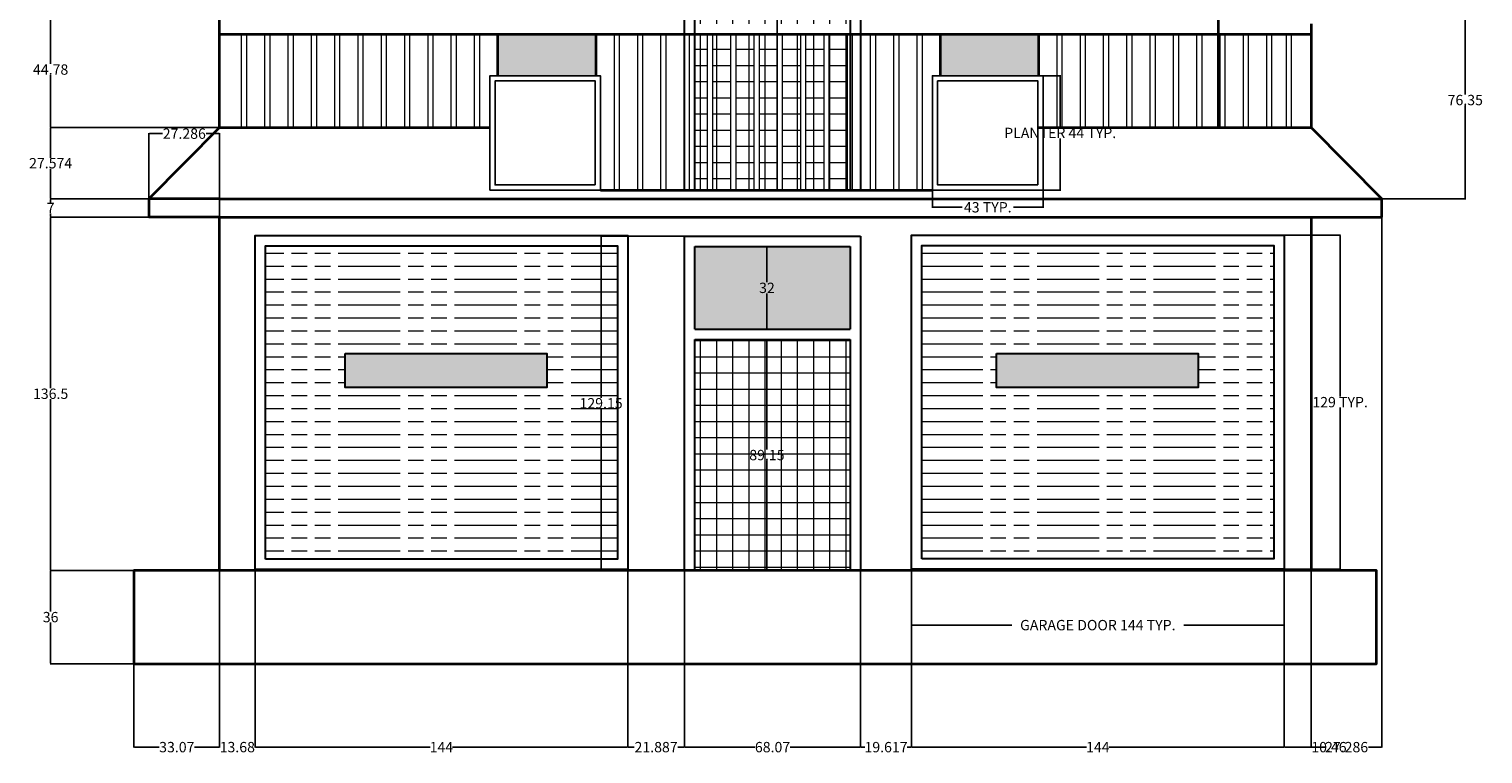
# Model space of a CAD drawing. Units: inches. Extents: x 1366 to 1929, y 372 to 1068.
# Tile 1 of 4: x 1366 to 1927, y 372 to 652. Entities that reach past the tile are written whole.
import ezdxf

# ---------------------------------------------------------------- set-up
doc = ezdxf.new("R2010")
doc.units = ezdxf.units.IN
doc.header["$MEASUREMENT"] = 0
for name, color, linetype, lineweight in [('A-ANNO-DIMS', 2, 'Continuous', 18), ('A-DOOR', 4, 'Continuous', 30), ('A-ELEV', 7, 'Continuous', 35), ('A-ELEV-PATT', 252, 'Continuous', 13), ('A-ELEV-PLNT', 3, 'Continuous', 25), ('A-ELEV-RAIL', 8, 'Continuous', 18)]:
    doc.layers.add(name, color=color, linetype=linetype, lineweight=lineweight)
doc.styles.get("Standard").update_dxf_attribs({"font": 'arial.ttf'})
doc.dimstyles.get("Standard").update_dxf_attribs({"dimtxt": 4, "dimasz": 0.18, "dimexe": 0.18, "dimexo": 0.0625, "dimgap": 0.09, "dimtad": 0, "dimtih": 1, "dimtoh": 1, "dimdec": 0, "dimrnd": 6, "dimzin": 0, "dimdsep": 46, "dimlunit": 3, "dimtxsty": 'Standard', "dimcen": 0.09, "dimadec": 0, "dimazin": 0, "dimtfac": 1, "dimtdec": 0, "dimtofl": 0, "dimtmove": 0, "dimatfit": 3, "dimfxl": 1, "dimtolj": 1, "dimtzin": 0, "dimarcsym": 0})

# ---------------------------------------------------------------- blocks, each defined once
blk = doc.blocks.new('GARAGE-DOOR')
for points in [[(0, 0), (0, 129), (144, 129), (144, 0)], [(4, 4), (4, 125), (140, 125), (140, 4)]]:
    blk.add_lwpolyline(points, close=True)
blk = doc.blocks.new('PLANTER')
for points in [[(42.71, 0), (0, 0), (0, 44.17), (42.71, 44.17)], [(40.71, 2), (2, 2), (2, 42.17), (40.71, 42.17)]]:
    blk.add_lwpolyline(points, close=True)
blk = doc.blocks.new('*D6')
at = {"layer": 'A-ANNO-DIMS', "color": 0, "lineweight": -2, "transparency": 16777216}
for p, q in [((1706.48, 442.89), (1706.48, 421.17)), ((1850.48, 442.89), (1850.48, 421.17)), ((1706.66, 421.35), (1745.24, 421.35)), ((1850.3, 421.35), (1811.71, 421.35))]:
    blk.add_line(p, q, dxfattribs=at)
at = {"layer": 'A-ANNO-DIMS', "color": 0, "lineweight": 30, "transparency": 16777216}
for points in [[(1706.66, 421.38), (1706.66, 421.32), (1706.48, 421.35)], [(1850.3, 421.38), (1850.3, 421.32), (1850.48, 421.35)]]:
    blk.add_solid(points, dxfattribs=at)
at = {"layer": 'Defpoints', "color": 0, "lineweight": 30, "transparency": 16777216}
for p in [(1706.48, 442.95), (1850.48, 442.95), (1850.48, 421.35)]:
    blk.add_point(p, dxfattribs=at)
at = {"layer": 'A-ANNO-DIMS', "color": 0, "transparency": 16777216, "insert": (1778.48, 421.35), "char_height": 4, "attachment_point": 5}
blk.add_mtext('\\A1;GARAGE DOOR 144 TYP.', dxfattribs=at)
blk = doc.blocks.new('*D7')
at = {"layer": 'A-ANNO-DIMS', "color": 0, "lineweight": -2, "transparency": 16777216}
for p, q in [((1850.54, 571.95), (1872.26, 571.95)), ((1872.08, 571.77), (1872.08, 509.59)), ((1872.08, 443.13), (1872.08, 505.32)), ((1850.54, 442.95), (1872.26, 442.95))]:
    blk.add_line(p, q, dxfattribs=at)
at = {"layer": 'A-ANNO-DIMS', "color": 0, "lineweight": 30, "transparency": 16777216}
for points in [[(1872.05, 571.77), (1872.11, 571.77), (1872.08, 571.95)], [(1872.05, 443.13), (1872.11, 443.13), (1872.08, 442.95)]]:
    blk.add_solid(points, dxfattribs=at)
at = {"layer": 'Defpoints', "color": 0, "lineweight": 30, "transparency": 16777216}
for p in [(1850.48, 571.95), (1872.08, 571.95), (1850.48, 442.95)]:
    blk.add_point(p, dxfattribs=at)
at = {"layer": 'A-ANNO-DIMS', "color": 0, "transparency": 16777216, "insert": (1872.08, 507.45), "char_height": 4, "attachment_point": 5}
blk.add_mtext('\\A1;129 TYP.', dxfattribs=at)
blk = doc.blocks.new('*D8')
at = {"layer": 'A-ANNO-DIMS', "color": 0, "lineweight": -2, "transparency": 16777216}
for p, q in [((1757.39, 633.5), (1764.13, 633.5)), ((1763.95, 633.32), (1763.95, 613.5)), ((1763.95, 589.5), (1763.95, 609.32)), ((1757.39, 589.32), (1764.13, 589.32))]:
    blk.add_line(p, q, dxfattribs=at)
at = {"layer": 'A-ANNO-DIMS', "color": 0, "lineweight": 30, "transparency": 16777216}
for points in [[(1763.92, 633.32), (1763.98, 633.32), (1763.95, 633.5)], [(1763.92, 589.5), (1763.98, 589.5), (1763.95, 589.32)]]:
    blk.add_solid(points, dxfattribs=at)
at = {"layer": 'Defpoints', "color": 0, "lineweight": 30, "transparency": 16777216}
for p in [(1757.32, 633.5), (1763.95, 633.5), (1757.32, 589.32)]:
    blk.add_point(p, dxfattribs=at)
at = {"layer": 'A-ANNO-DIMS', "color": 0, "transparency": 16777216, "insert": (1763.95, 611.41), "char_height": 4, "attachment_point": 5}
blk.add_mtext('\\A1;PLANTER 44 TYP.', dxfattribs=at)
blk = doc.blocks.new('*D9')
at = {"layer": 'A-ANNO-DIMS', "color": 0, "lineweight": -2, "transparency": 16777216}
for p, q in [((1714.61, 589.26), (1714.61, 582.52)), ((1757.32, 589.26), (1757.32, 582.52)), ((1714.79, 582.7), (1726.06, 582.7)), ((1757.14, 582.7), (1745.87, 582.7))]:
    blk.add_line(p, q, dxfattribs=at)
at = {"layer": 'A-ANNO-DIMS', "color": 0, "lineweight": 30, "transparency": 16777216}
for points in [[(1714.79, 582.73), (1714.79, 582.67), (1714.61, 582.7)], [(1757.14, 582.73), (1757.14, 582.67), (1757.32, 582.7)]]:
    blk.add_solid(points, dxfattribs=at)
at = {"layer": 'Defpoints', "color": 0, "lineweight": 30, "transparency": 16777216}
for p in [(1714.61, 589.32), (1757.32, 589.32), (1757.32, 582.7)]:
    blk.add_point(p, dxfattribs=at)
at = {"layer": 'A-ANNO-DIMS', "color": 0, "transparency": 16777216, "insert": (1735.97, 582.7), "char_height": 4, "attachment_point": 5}
blk.add_mtext('\\A1;43 TYP.', dxfattribs=at)
blk = doc.blocks.new('*D18')
at = {"layer": 'A-ANNO-DIMS', "color": 0, "lineweight": -2, "transparency": 16777216}
for p, q in [((1439.22, 442.38), (1439.22, 374.06)), ((1406.15, 406.38), (1406.15, 374.06)), ((1406.33, 374.24), (1415.85, 374.24)), ((1439.04, 374.24), (1429.52, 374.24))]:
    blk.add_line(p, q, dxfattribs=at)
at = {"layer": 'A-ANNO-DIMS', "color": 0, "lineweight": 30, "transparency": 16777216}
for points in [[(1406.33, 374.27), (1406.33, 374.21), (1406.15, 374.24)], [(1439.04, 374.27), (1439.04, 374.21), (1439.22, 374.24)]]:
    blk.add_solid(points, dxfattribs=at)
at = {"layer": 'Defpoints', "color": 0, "lineweight": 30, "transparency": 16777216}
for p in [(1439.22, 442.44), (1406.15, 406.44), (1439.22, 374.24)]:
    blk.add_point(p, dxfattribs=at)
at = {"layer": 'A-ANNO-DIMS', "color": 0, "transparency": 16777216, "insert": (1422.69, 374.24), "char_height": 4, "attachment_point": 5}
blk.add_mtext('\\A1;33.07', dxfattribs=at)
blk = doc.blocks.new('*D19')
at = {"layer": 'A-ANNO-DIMS', "color": 0, "lineweight": -2, "transparency": 16777216}
for p, q in [((1439.221801, 442.38172), (1439.221801, 374.06422)), ((1452.900921, 442.704563), (1452.900921, 374.06422)), ((1439.041801, 374.24422), (1438.861801, 374.24422)), ((1453.080921, 374.24422), (1453.260921, 374.24422))]:
    blk.add_line(p, q, dxfattribs=at)
at = {"layer": 'A-ANNO-DIMS', "color": 0, "lineweight": 30, "transparency": 16777216}
for points in [[(1439.041801, 374.27422), (1439.041801, 374.21422), (1439.221801, 374.24422)], [(1453.080921, 374.27422), (1453.080921, 374.21422), (1452.900921, 374.24422)]]:
    blk.add_solid(points, dxfattribs=at)
at = {"layer": 'Defpoints', "color": 0, "lineweight": 30, "transparency": 16777216}
for p in [(1439.221801, 442.44422), (1452.900921, 442.767063), (1452.900921, 374.24422)]:
    blk.add_point(p, dxfattribs=at)
at = {"layer": 'A-ANNO-DIMS', "color": 0, "transparency": 16777216, "insert": (1446.061361, 374.24422), "char_height": 4, "attachment_point": 5}
blk.add_mtext('\\A1;13.68', dxfattribs=at)
blk = doc.blocks.new('*D20')
at = {"layer": 'A-ANNO-DIMS', "color": 0, "lineweight": -2, "transparency": 16777216}
for p, q in [((1452.9, 442.7), (1452.9, 374.06)), ((1596.9, 442.7), (1596.9, 374.06)), ((1453.08, 374.24), (1520.59, 374.24)), ((1596.72, 374.24), (1529.21, 374.24))]:
    blk.add_line(p, q, dxfattribs=at)
at = {"layer": 'A-ANNO-DIMS', "color": 0, "lineweight": 30, "transparency": 16777216}
for points in [[(1453.08, 374.27), (1453.08, 374.21), (1452.9, 374.24)], [(1596.72, 374.27), (1596.72, 374.21), (1596.9, 374.24)]]:
    blk.add_solid(points, dxfattribs=at)
at = {"layer": 'Defpoints', "color": 0, "lineweight": 30, "transparency": 16777216}
for p in [(1452.9, 442.77), (1596.9, 442.77), (1596.9, 374.24)]:
    blk.add_point(p, dxfattribs=at)
at = {"layer": 'A-ANNO-DIMS', "color": 0, "transparency": 16777216, "insert": (1524.9, 374.24), "char_height": 4, "attachment_point": 5}
blk.add_mtext('\\A1;144', dxfattribs=at)
blk = doc.blocks.new('*D21')
at = {"layer": 'A-ANNO-DIMS', "color": 0, "lineweight": -2, "transparency": 16777216}
for p, q in [((1596.9, 442.7), (1596.9, 374.06)), ((1618.79, 442.38), (1618.79, 374.06)), ((1597.08, 374.24), (1599.42, 374.24)), ((1618.61, 374.24), (1616.27, 374.24))]:
    blk.add_line(p, q, dxfattribs=at)
at = {"layer": 'A-ANNO-DIMS', "color": 0, "lineweight": 30, "transparency": 16777216}
for points in [[(1597.08, 374.27), (1597.08, 374.21), (1596.9, 374.24)], [(1618.61, 374.27), (1618.61, 374.21), (1618.79, 374.24)]]:
    blk.add_solid(points, dxfattribs=at)
at = {"layer": 'Defpoints', "color": 0, "lineweight": 30, "transparency": 16777216}
for p in [(1596.9, 442.77), (1618.79, 442.44), (1618.79, 374.24)]:
    blk.add_point(p, dxfattribs=at)
at = {"layer": 'A-ANNO-DIMS', "color": 0, "transparency": 16777216, "insert": (1607.84, 374.24), "char_height": 4, "attachment_point": 5}
blk.add_mtext('\\A1;21.887', dxfattribs=at)
blk = doc.blocks.new('*D22')
at = {"layer": 'A-ANNO-DIMS', "color": 0, "lineweight": -2, "transparency": 16777216}
for p, q in [((1618.79, 442.38), (1618.79, 374.06)), ((1686.86, 442.38), (1686.86, 374.06)), ((1618.97, 374.24), (1645.97, 374.24)), ((1686.68, 374.24), (1659.67, 374.24))]:
    blk.add_line(p, q, dxfattribs=at)
at = {"layer": 'A-ANNO-DIMS', "color": 0, "lineweight": 30, "transparency": 16777216}
for points in [[(1618.97, 374.27), (1618.97, 374.21), (1618.79, 374.24)], [(1686.68, 374.27), (1686.68, 374.21), (1686.86, 374.24)]]:
    blk.add_solid(points, dxfattribs=at)
at = {"layer": 'Defpoints', "color": 0, "lineweight": 30, "transparency": 16777216}
for p in [(1618.79, 442.44), (1686.86, 442.44), (1686.86, 374.24)]:
    blk.add_point(p, dxfattribs=at)
at = {"layer": 'A-ANNO-DIMS', "color": 0, "transparency": 16777216, "insert": (1652.82, 374.24), "char_height": 4, "attachment_point": 5}
blk.add_mtext('\\A1;68.07', dxfattribs=at)
blk = doc.blocks.new('*D23')
at = {"layer": 'A-ANNO-DIMS', "color": 0, "lineweight": -2, "transparency": 16777216}
for p, q in [((1686.86, 442.38), (1686.86, 374.06)), ((1706.48, 442.89), (1706.48, 374.06)), ((1687.04, 374.24), (1688.46, 374.24)), ((1706.3, 374.24), (1704.87, 374.24))]:
    blk.add_line(p, q, dxfattribs=at)
at = {"layer": 'A-ANNO-DIMS', "color": 0, "lineweight": 30, "transparency": 16777216}
for points in [[(1687.04, 374.27), (1687.04, 374.21), (1686.86, 374.24)], [(1706.3, 374.27), (1706.3, 374.21), (1706.48, 374.24)]]:
    blk.add_solid(points, dxfattribs=at)
at = {"layer": 'Defpoints', "color": 0, "lineweight": 30, "transparency": 16777216}
for p in [(1686.86, 442.44), (1706.48, 442.95), (1706.48, 374.24)]:
    blk.add_point(p, dxfattribs=at)
at = {"layer": 'A-ANNO-DIMS', "color": 0, "transparency": 16777216, "insert": (1696.67, 374.24), "char_height": 4, "attachment_point": 5}
blk.add_mtext('\\A1;19.617', dxfattribs=at)
blk = doc.blocks.new('*D24')
at = {"layer": 'A-ANNO-DIMS', "color": 0, "lineweight": -2, "transparency": 16777216}
for p, q in [((1706.48, 442.89), (1706.48, 374.06)), ((1850.48, 442.89), (1850.48, 374.06)), ((1706.66, 374.24), (1774.16, 374.24)), ((1850.3, 374.24), (1782.79, 374.24))]:
    blk.add_line(p, q, dxfattribs=at)
at = {"layer": 'A-ANNO-DIMS', "color": 0, "lineweight": 30, "transparency": 16777216}
for points in [[(1706.66, 374.27), (1706.66, 374.21), (1706.48, 374.24)], [(1850.3, 374.27), (1850.3, 374.21), (1850.48, 374.24)]]:
    blk.add_solid(points, dxfattribs=at)
at = {"layer": 'Defpoints', "color": 0, "lineweight": 30, "transparency": 16777216}
for p in [(1706.48, 442.95), (1850.48, 442.95), (1850.48, 374.24)]:
    blk.add_point(p, dxfattribs=at)
at = {"layer": 'A-ANNO-DIMS', "color": 0, "transparency": 16777216, "insert": (1778.48, 374.24), "char_height": 4, "attachment_point": 5}
blk.add_mtext('\\A1;144', dxfattribs=at)
blk = doc.blocks.new('*D25')
at = {"layer": 'A-ANNO-DIMS', "color": 0, "lineweight": -2, "transparency": 16777216}
for p, q in [((1850.48, 442.89), (1850.48, 374.06)), ((1860.94, 442.38), (1860.94, 374.06)), ((1850.66, 374.24), (1860.76, 374.24)), ((1860.94, 374.24), (1861.12, 374.24))]:
    blk.add_line(p, q, dxfattribs=at)
at = {"layer": 'A-ANNO-DIMS', "color": 0, "lineweight": 30, "transparency": 16777216}
for points in [[(1850.66, 374.27), (1850.66, 374.21), (1850.48, 374.24)], [(1860.76, 374.27), (1860.76, 374.21), (1860.94, 374.24)]]:
    blk.add_solid(points, dxfattribs=at)
at = {"layer": 'Defpoints', "color": 0, "lineweight": 30, "transparency": 16777216}
for p in [(1850.48, 442.95), (1860.94, 442.44), (1860.94, 374.24)]:
    blk.add_point(p, dxfattribs=at)
at = {"layer": 'A-ANNO-DIMS', "color": 0, "transparency": 16777216, "insert": (1867.76, 374.24), "char_height": 4, "attachment_point": 5}
blk.add_mtext('\\A1;10.46', dxfattribs=at)
blk = doc.blocks.new('*D26')
at = {"layer": 'A-ANNO-DIMS', "color": 0, "lineweight": -2, "transparency": 16777216}
for p, q in [((1888.22, 585.87), (1888.22, 374.06)), ((1860.94, 442.38), (1860.94, 374.06)), ((1861.12, 374.24), (1866.15, 374.24)), ((1888.04, 374.24), (1883, 374.24))]:
    blk.add_line(p, q, dxfattribs=at)
at = {"layer": 'A-ANNO-DIMS', "color": 0, "lineweight": 30, "transparency": 16777216}
for points in [[(1861.12, 374.27), (1861.12, 374.21), (1860.94, 374.24)], [(1888.04, 374.27), (1888.04, 374.21), (1888.22, 374.24)]]:
    blk.add_solid(points, dxfattribs=at)
at = {"layer": 'Defpoints', "color": 0, "lineweight": 30, "transparency": 16777216}
for p in [(1888.22, 585.93), (1860.94, 442.44), (1888.22, 374.24)]:
    blk.add_point(p, dxfattribs=at)
at = {"layer": 'A-ANNO-DIMS', "color": 0, "transparency": 16777216, "insert": (1874.58, 374.24), "char_height": 4, "attachment_point": 5}
blk.add_mtext('\\A1;27.286', dxfattribs=at)
blk = doc.blocks.new('*D27')
at = {"layer": 'A-ANNO-DIMS', "color": 0, "lineweight": -2, "transparency": 16777216}
for p, q in [((1406.09, 442.44), (1373.77, 442.44)), ((1373.95, 442.26), (1373.95, 426.58)), ((1373.95, 406.62), (1373.95, 422.31)), ((1406.09, 406.44), (1373.77, 406.44))]:
    blk.add_line(p, q, dxfattribs=at)
at = {"layer": 'A-ANNO-DIMS', "color": 0, "lineweight": 30, "transparency": 16777216}
for points in [[(1373.92, 442.26), (1373.98, 442.26), (1373.95, 442.44)], [(1373.92, 406.62), (1373.98, 406.62), (1373.95, 406.44)]]:
    blk.add_solid(points, dxfattribs=at)
at = {"layer": 'Defpoints', "color": 0, "lineweight": 30, "transparency": 16777216}
for p in [(1373.95, 442.44), (1406.15, 442.44), (1406.15, 406.44)]:
    blk.add_point(p, dxfattribs=at)
at = {"layer": 'A-ANNO-DIMS', "color": 0, "transparency": 16777216, "insert": (1373.95, 424.44), "char_height": 4, "attachment_point": 5}
blk.add_mtext('\\A1;36', dxfattribs=at)
blk = doc.blocks.new('*D28')
at = {"layer": 'A-ANNO-DIMS', "color": 0, "lineweight": -2, "transparency": 16777216}
for p, q in [((1439.16, 578.93), (1373.77, 578.93)), ((1373.95, 578.75), (1373.95, 512.82)), ((1373.95, 442.62), (1373.95, 508.55)), ((1406.09, 442.44), (1373.77, 442.44))]:
    blk.add_line(p, q, dxfattribs=at)
at = {"layer": 'A-ANNO-DIMS', "color": 0, "lineweight": 30, "transparency": 16777216}
for points in [[(1373.92, 578.75), (1373.98, 578.75), (1373.95, 578.93)], [(1373.92, 442.62), (1373.98, 442.62), (1373.95, 442.44)]]:
    blk.add_solid(points, dxfattribs=at)
at = {"layer": 'Defpoints', "color": 0, "lineweight": 30, "transparency": 16777216}
for p in [(1373.95, 578.93), (1439.22, 578.93), (1406.15, 442.44)]:
    blk.add_point(p, dxfattribs=at)
at = {"layer": 'A-ANNO-DIMS', "color": 0, "transparency": 16777216, "insert": (1373.95, 510.69), "char_height": 4, "attachment_point": 5}
blk.add_mtext('\\A1;136.5', dxfattribs=at)
blk = doc.blocks.new('*D29')
at = {"layer": 'A-ANNO-DIMS', "color": 0, "lineweight": -2, "transparency": 16777216}
for p, q in [((1411.87353, 585.931246), (1373.772656, 585.931246)), ((1373.952656, 585.751246), (1373.952656, 584.521246)), ((1439.159301, 578.931246), (1373.772656, 578.931246)), ((1373.952656, 579.111246), (1373.952656, 580.341246))]:
    blk.add_line(p, q, dxfattribs=at)
at = {"layer": 'A-ANNO-DIMS', "color": 0, "lineweight": 30, "transparency": 16777216}
for points in [[(1373.922656, 585.751246), (1373.982656, 585.751246), (1373.952656, 585.931246)], [(1373.922656, 579.111246), (1373.982656, 579.111246), (1373.952656, 578.931246)]]:
    blk.add_solid(points, dxfattribs=at)
at = {"layer": 'Defpoints', "color": 0, "lineweight": 30, "transparency": 16777216}
for p in [(1373.952656, 585.931246), (1411.93603, 585.931246), (1439.221801, 578.931246)]:
    blk.add_point(p, dxfattribs=at)
at = {"layer": 'A-ANNO-DIMS', "color": 0, "transparency": 16777216, "insert": (1373.952656, 582.431246), "char_height": 4, "attachment_point": 5}
blk.add_mtext('\\A1;7', dxfattribs=at)
blk = doc.blocks.new('*D30')
at = {"layer": 'A-ANNO-DIMS', "color": 0, "lineweight": -2, "transparency": 16777216}
for p, q in [((1439.16, 613.51), (1373.77, 613.51)), ((1373.95, 613.33), (1373.95, 601.85)), ((1373.95, 586.11), (1373.95, 597.59)), ((1411.87, 585.93), (1373.77, 585.93))]:
    blk.add_line(p, q, dxfattribs=at)
at = {"layer": 'A-ANNO-DIMS', "color": 0, "lineweight": 30, "transparency": 16777216}
for points in [[(1373.92, 613.33), (1373.98, 613.33), (1373.95, 613.51)], [(1373.92, 586.11), (1373.98, 586.11), (1373.95, 585.93)]]:
    blk.add_solid(points, dxfattribs=at)
at = {"layer": 'Defpoints', "color": 0, "lineweight": 30, "transparency": 16777216}
for p in [(1373.95, 613.51), (1439.22, 613.51), (1411.94, 585.93)]:
    blk.add_point(p, dxfattribs=at)
at = {"layer": 'A-ANNO-DIMS', "color": 0, "transparency": 16777216, "insert": (1373.95, 599.72), "char_height": 4, "attachment_point": 5}
blk.add_mtext('\\A1;27.574', dxfattribs=at)
blk = doc.blocks.new('*D31')
at = {"layer": 'A-ANNO-DIMS', "color": 0, "lineweight": -2, "transparency": 16777216}
for p, q in [((1466.76, 658.28), (1373.77, 658.28)), ((1373.95, 658.1), (1373.95, 638.03)), ((1373.95, 613.69), (1373.95, 633.76)), ((1439.16, 613.51), (1373.77, 613.51))]:
    blk.add_line(p, q, dxfattribs=at)
at = {"layer": 'A-ANNO-DIMS', "color": 0, "lineweight": 30, "transparency": 16777216}
for points in [[(1373.92, 658.1), (1373.98, 658.1), (1373.95, 658.28)], [(1373.92, 613.69), (1373.98, 613.69), (1373.95, 613.51)]]:
    blk.add_solid(points, dxfattribs=at)
at = {"layer": 'Defpoints', "color": 0, "lineweight": 30, "transparency": 16777216}
for p in [(1373.95, 658.28), (1466.83, 658.28), (1439.22, 613.51)]:
    blk.add_point(p, dxfattribs=at)
at = {"layer": 'A-ANNO-DIMS', "color": 0, "transparency": 16777216, "insert": (1373.95, 635.89), "char_height": 4, "attachment_point": 5}
blk.add_mtext('\\A1;44.78', dxfattribs=at)
blk = doc.blocks.new('*D43')
at = {"layer": 'A-ANNO-DIMS', "color": 0, "lineweight": -2, "transparency": 16777216}
for p, q in [((1820.78, 662.28), (1920.61, 662.28)), ((1920.43, 662.1), (1920.43, 626.24)), ((1920.43, 586.11), (1920.43, 621.97)), ((1888.28, 585.93), (1920.61, 585.93))]:
    blk.add_line(p, q, dxfattribs=at)
at = {"layer": 'A-ANNO-DIMS', "color": 0, "lineweight": 30, "transparency": 16777216}
for points in [[(1920.4, 662.1), (1920.46, 662.1), (1920.43, 662.28)], [(1920.4, 586.11), (1920.46, 586.11), (1920.43, 585.93)]]:
    blk.add_solid(points, dxfattribs=at)
at = {"layer": 'Defpoints', "color": 0, "lineweight": 30, "transparency": 16777216}
for p in [(1820.72, 662.28), (1920.43, 662.28), (1888.22, 585.93)]:
    blk.add_point(p, dxfattribs=at)
at = {"layer": 'A-ANNO-DIMS', "color": 0, "transparency": 16777216, "insert": (1920.43, 624.11), "char_height": 4, "attachment_point": 5}
blk.add_mtext('\\A1;76.35', dxfattribs=at)
blk = doc.blocks.new('*D54')
at = {"layer": 'A-ANNO-DIMS', "color": 0, "lineweight": -2, "transparency": 16777216}
for p, q in [((1411.94, 578.99), (1411.94, 611.31)), ((1412.12, 611.13), (1417.15, 611.13)), ((1439.04, 611.13), (1434, 611.13)), ((1439.22, 578.99), (1439.22, 611.31))]:
    blk.add_line(p, q, dxfattribs=at)
at = {"layer": 'A-ANNO-DIMS', "color": 0, "lineweight": 30, "transparency": 16777216}
for points in [[(1412.12, 611.16), (1412.12, 611.1), (1411.94, 611.13)], [(1439.04, 611.16), (1439.04, 611.1), (1439.22, 611.13)]]:
    blk.add_solid(points, dxfattribs=at)
at = {"layer": 'Defpoints', "color": 0, "lineweight": 30, "transparency": 16777216}
for p in [(1439.22, 611.13), (1411.94, 578.93), (1439.22, 578.93)]:
    blk.add_point(p, dxfattribs=at)
at = {"layer": 'A-ANNO-DIMS', "color": 0, "transparency": 16777216, "insert": (1425.58, 611.13), "char_height": 4, "attachment_point": 5}
blk.add_mtext('\\A1;27.286', dxfattribs=at)
blk = doc.blocks.new('*D58')
at = {"layer": 'A-ANNO-DIMS', "color": 0, "lineweight": -2, "transparency": 16777216}
for p, q in [((1618.73, 571.59), (1586.41, 571.59)), ((1586.59, 571.41), (1586.59, 509.15)), ((1586.59, 442.62), (1586.59, 504.89)), ((1618.73, 442.44), (1586.41, 442.44))]:
    blk.add_line(p, q, dxfattribs=at)
at = {"layer": 'A-ANNO-DIMS', "color": 0, "lineweight": 30, "transparency": 16777216}
for points in [[(1586.56, 571.41), (1586.62, 571.41), (1586.59, 571.59)], [(1586.56, 442.62), (1586.62, 442.62), (1586.59, 442.44)]]:
    blk.add_solid(points, dxfattribs=at)
at = {"layer": 'Defpoints', "color": 0, "lineweight": 30, "transparency": 16777216}
for p in [(1586.59, 571.59), (1618.79, 571.59), (1618.79, 442.44)]:
    blk.add_point(p, dxfattribs=at)
at = {"layer": 'A-ANNO-DIMS', "color": 0, "transparency": 16777216, "insert": (1586.59, 507.02), "char_height": 4, "attachment_point": 5}
blk.add_mtext('\\A1;129.15', dxfattribs=at)
blk = doc.blocks.new('*D59')
at = {"layer": 'A-ANNO-DIMS', "color": 0, "lineweight": -2, "transparency": 16777216}
for p, q in [((1682.8, 567.59), (1650.48, 567.59)), ((1650.66, 567.41), (1650.66, 553.73)), ((1650.66, 535.77), (1650.66, 549.46)), ((1682.8, 535.59), (1650.48, 535.59))]:
    blk.add_line(p, q, dxfattribs=at)
at = {"layer": 'A-ANNO-DIMS', "color": 0, "lineweight": 30, "transparency": 16777216}
for points in [[(1650.63, 567.41), (1650.69, 567.41), (1650.66, 567.59)], [(1650.63, 535.77), (1650.69, 535.77), (1650.66, 535.59)]]:
    blk.add_solid(points, dxfattribs=at)
at = {"layer": 'Defpoints', "color": 0, "lineweight": 30, "transparency": 16777216}
for p in [(1650.66, 567.59), (1682.86, 567.59), (1682.86, 535.59)]:
    blk.add_point(p, dxfattribs=at)
at = {"layer": 'A-ANNO-DIMS', "color": 0, "transparency": 16777216, "insert": (1650.66, 551.59), "char_height": 4, "attachment_point": 5}
blk.add_mtext('\\A1;32', dxfattribs=at)
blk = doc.blocks.new('*D60')
at = {"layer": 'A-ANNO-DIMS', "color": 0, "lineweight": -2, "transparency": 16777216}
for p, q in [((1682.8, 531.59), (1650.48, 531.59)), ((1650.66, 531.41), (1650.66, 489.15)), ((1650.66, 442.62), (1650.66, 484.89)), ((1682.8, 442.44), (1650.48, 442.44))]:
    blk.add_line(p, q, dxfattribs=at)
at = {"layer": 'A-ANNO-DIMS', "color": 0, "lineweight": 30, "transparency": 16777216}
for points in [[(1650.63, 531.41), (1650.69, 531.41), (1650.66, 531.59)], [(1650.63, 442.62), (1650.69, 442.62), (1650.66, 442.44)]]:
    blk.add_solid(points, dxfattribs=at)
at = {"layer": 'Defpoints', "color": 0, "lineweight": 30, "transparency": 16777216}
for p in [(1650.66, 531.59), (1682.86, 531.59), (1682.86, 442.44)]:
    blk.add_point(p, dxfattribs=at)
at = {"layer": 'A-ANNO-DIMS', "color": 0, "transparency": 16777216, "insert": (1650.66, 487.02), "char_height": 4, "attachment_point": 5}
blk.add_mtext('\\A1;89.15', dxfattribs=at)
blk = doc.blocks.new('*D61')
at = {"layer": 'A-ANNO-DIMS', "color": 0, "lineweight": -2, "transparency": 16777216}
for p, q in [((1686.8, 743.18), (1654.48, 743.18)), ((1654.66, 743), (1654.66, 668.38)), ((1654.66, 589.5), (1654.66, 664.12)), ((1686.8, 589.32), (1654.48, 589.32))]:
    blk.add_line(p, q, dxfattribs=at)
at = {"layer": 'A-ANNO-DIMS', "color": 0, "lineweight": 30, "transparency": 16777216}
for points in [[(1654.63, 743), (1654.69, 743), (1654.66, 743.18)], [(1654.63, 589.5), (1654.69, 589.5), (1654.66, 589.32)]]:
    blk.add_solid(points, dxfattribs=at)
at = {"layer": 'Defpoints', "color": 0, "lineweight": 30, "transparency": 16777216}
for p in [(1654.66, 743.18), (1686.86, 743.18), (1686.86, 589.32)]:
    blk.add_point(p, dxfattribs=at)
at = {"layer": 'A-ANNO-DIMS', "color": 0, "transparency": 16777216, "insert": (1654.66, 666.25), "char_height": 4, "attachment_point": 5}
blk.add_mtext('\\A1;153.85', dxfattribs=at)

msp = doc.modelspace()

# ---------------------------------------------------------------- hatches: boundary and pattern name
at = {"layer": 'A-ELEV-PATT'}
h = msp.add_hatch(dxfattribs=at)
h.set_pattern_fill('ANGLE', color=256, scale=25)
h.set_pattern_definition([(0, (0, 0), (0, 6.875), [5, -1.875]), (90, (0, 0), (-6.875, 4e-16), [5, -1.875])])
h.paths.add_polyline_path([(1544.6356, 893.5665), (1508.6356, 893.5665), (1508.6356, 828.2264), (1544.6356, 828.2264)])
h.paths.add_polyline_path([(1506.6356, 727.6227), (1470.827, 727.6227), (1470.827, 662.2826), (1506.6356, 662.2826)])
h.paths.add_polyline_path([(1544.6356, 727.6227), (1508.6356, 727.6227), (1508.6356, 662.2826), (1544.6356, 662.2826)])
h.paths.add_polyline_path([(1608.5338, 752.9927), (1697.2248, 752.9927, 0.93463511)])
h.paths.add_polyline_path([(1682.8585, 567.593), (1622.7881, 567.593), (1622.7881, 535.593), (1682.8585, 535.593)])
h.paths.add_polyline_path([(1782.7172, 723.6227), (1750.9085, 723.6227), (1750.9085, 666.2826), (1782.7172, 666.2826)])
h.paths.add_polyline_path([(1816.7172, 723.6227), (1784.7172, 723.6227), (1784.7172, 666.2826), (1816.7172, 666.2826)])
h.paths.add_polyline_path([(1817.1901, 526.1862), (1739.2847, 526.1862), (1739.2847, 513.1136), (1817.1901, 513.1136)])
h.paths.add_polyline_path([(1565.633, 526.1862), (1487.7276, 526.1862), (1487.7276, 513.1136), (1565.633, 513.1136)])
h = msp.add_hatch(dxfattribs=at)
h.set_pattern_fill('NET', color=256, scale=50)
h.paths.add_polyline_path([(1682.8585, 739.1753), (1622.7881, 739.1753), (1622.7881, 653.5057), (1682.8585, 653.5057)])
h.paths.add_polyline_path([(1682.8585, 531.593), (1622.7881, 531.593), (1622.7881, 442.4442), (1682.8585, 442.4442)])
h.paths.add_polyline_path([(1627.6001, 649.5057), (1622.7881, 649.5057), (1622.7881, 589.3234), (1627.6001, 589.3234)])
h.paths.add_polyline_path([(1636.6001, 649.5057), (1629.6001, 649.5057), (1629.6001, 589.3234), (1636.6001, 589.3234)])
h.paths.add_polyline_path([(1645.6001, 649.5057), (1638.6001, 649.5057), (1638.6001, 589.3234), (1645.6001, 589.3234)])
h.paths.add_polyline_path([(1654.6001, 649.5057), (1647.6001, 649.5057), (1647.6001, 589.3234), (1654.6001, 589.3234)])
h.paths.add_polyline_path([(1663.6001, 649.5057), (1656.6001, 649.5057), (1656.6001, 589.3234), (1663.6001, 589.3234)])
h.paths.add_polyline_path([(1672.6001, 649.5057), (1665.6001, 649.5057), (1665.6001, 589.3234), (1672.6001, 589.3234)])
h.paths.add_polyline_path([(1681.6001, 649.5057), (1674.6001, 649.5057), (1674.6001, 589.3234), (1681.6001, 589.3234)])
h = msp.add_hatch(dxfattribs=at)
h.set_pattern_fill('ESCHER', color=256, scale=5)
h.paths.add_polyline_path([(1584.6001, 649.5057), (1546.6001, 649.5057), (1546.6001, 633.4977), (1584.6001, 633.4977)])
h.paths.add_polyline_path([(1755.6001, 649.5057), (1717.6001, 649.5057), (1717.6001, 633.4977), (1755.6001, 633.4977)])
h = msp.add_hatch(dxfattribs=at)
h.set_pattern_fill('ACAD_ISO09W100', color=256)
h.set_pattern_definition([(0, (0, 0), (0, 5), [24, -3, 6, -3, 6, -3])])
h.paths.add_polyline_path([(1592.9009, 567.7671), (1456.9009, 567.7671), (1456.9009, 446.7671), (1592.9009, 446.7671)])
h.paths.add_polyline_path([(1487.7276, 513.1136), (1487.7276, 526.1862), (1565.633, 526.1862), (1565.633, 513.1136)], flags=16)
h.paths.add_polyline_path([(1846.4756, 567.9544), (1710.4756, 567.9544), (1710.4756, 446.9544), (1846.4756, 446.9544)])
h.paths.add_polyline_path([(1739.2847, 513.1136), (1739.2847, 526.1862), (1817.1901, 526.1862), (1817.1901, 513.1136)], flags=16)

# ---------------------------------------------------------------- linework, layer by layer
at = {"layer": 'A-DOOR'}
for p, q in [((1618.7881, 571.593), (1686.8585, 571.593)), ((1618.7881, 442.4442), (1618.7881, 571.593)), ((1622.7881, 567.593), (1682.8585, 567.593)), ((1622.7881, 535.593), (1622.7881, 567.593)), ((1682.8585, 567.593), (1682.8585, 535.593)), ((1686.8585, 571.593), (1686.8585, 442.4442)), ((1622.7881, 535.593), (1682.8585, 535.593)), ((1622.7881, 442.4442), (1622.7881, 531.593)), ((1622.7881, 531.593), (1682.8585, 531.593)), ((1682.8585, 531.593), (1682.8585, 442.4442))]:
    msp.add_line(p, q, dxfattribs=at)
for points in [[(1618.7881, 589.3234), (1618.7881, 743.1753), (1686.8585, 743.1753), (1686.8585, 589.3234)], [(1622.7881, 589.3234), (1622.7881, 739.1753), (1682.8585, 739.1753), (1682.8585, 589.3234)]]:
    msp.add_lwpolyline(points, dxfattribs=at)
for points in [[(1487.7276, 526.1862), (1565.633, 526.1862), (1565.633, 513.1136), (1487.7276, 513.1136)], [(1739.2847, 526.1862), (1817.1901, 526.1862), (1817.1901, 513.1136), (1739.2847, 513.1136)]]:
    msp.add_lwpolyline(points, close=True, dxfattribs=at)
at = {"layer": 'A-ELEV'}
for p, q in [((1439.2218, 613.5057), (1439.2218, 749.9927)), ((1824.9351, 749.9927), (1824.9351, 613.5057)), ((1860.9351, 653.5057), (1860.9351, 613.5057)), ((1439.2218, 649.5057), (1860.9351, 649.5057)), ((1546.6001, 649.5057), (1546.6001, 633.4977)), ((1584.6001, 649.5057), (1584.6001, 633.4977)), ((1717.6001, 649.5057), (1717.6001, 633.4977)), ((1755.6001, 649.5057), (1755.6001, 633.4977)), ((1439.2218, 613.5057), (1411.936, 585.9312)), ((1439.2218, 613.5057), (1543.6464, 613.5057)), ((1755.3233, 613.5057), (1860.9351, 613.5057)), ((1860.9351, 613.5057), (1888.2208, 585.9312)), ((1439.2218, 585.9312), (1411.936, 585.9312)), ((1411.936, 585.9312), (1411.936, 578.9312)), ((1439.2218, 585.9312), (1860.9351, 585.9312)), ((1586.3581, 589.3234), (1714.6115, 589.3234)), ((1860.9351, 585.9312), (1888.2208, 585.9312)), ((1888.2297, 578.9312), (1888.2208, 585.9312)), ((1439.2218, 578.9312), (1411.936, 578.9312)), ((1439.2218, 442.4442), (1439.2218, 578.9312)), ((1439.2218, 578.9312), (1860.9351, 578.9312)), ((1860.9351, 578.9312), (1860.9351, 442.4442)), ((1860.9351, 578.9312), (1888.2297, 578.9312))]:
    msp.add_line(p, q, dxfattribs=at)
msp.add_lwpolyline([(1406.1527, 406.4442), (1886.1527, 406.4442), (1886.1527, 442.4442), (1406.1527, 442.4442)], close=True, dxfattribs=at)
at = {"layer": 'A-ELEV-RAIL'}
for p, q in [((1447.6001, 649.5057), (1447.6001, 613.5057)), ((1449.6001, 649.5057), (1449.6001, 613.5057)), ((1456.6001, 649.5057), (1456.6001, 613.5057)), ((1458.6001, 649.5057), (1458.6001, 613.5057)), ((1465.6001, 649.5057), (1465.6001, 613.5057)), ((1467.6001, 649.5057), (1467.6001, 613.5057)), ((1474.6001, 649.5057), (1474.6001, 613.5057)), ((1476.6001, 649.5057), (1476.6001, 613.5057)), ((1483.6001, 649.5057), (1483.6001, 613.5057)), ((1485.6001, 649.5057), (1485.6001, 613.5057)), ((1492.6001, 649.5057), (1492.6001, 613.5057)), ((1494.6001, 649.5057), (1494.6001, 613.5057)), ((1501.6001, 649.5057), (1501.6001, 613.5057)), ((1503.6001, 649.5057), (1503.6001, 613.5057)), ((1510.6001, 649.5057), (1510.6001, 613.5057)), ((1512.6001, 649.5057), (1512.6001, 613.5057)), ((1519.6001, 649.5057), (1519.6001, 613.5057)), ((1521.6001, 649.5057), (1521.6001, 613.5057)), ((1528.6001, 649.5057), (1528.6001, 613.5057)), ((1530.6001, 649.5057), (1530.6001, 613.5057)), ((1537.6001, 649.5057), (1537.6001, 613.5057)), ((1539.6001, 649.5057), (1539.6001, 613.5057)), ((1591.6001, 649.5057), (1591.6001, 589.3234)), ((1593.6001, 649.5057), (1593.6001, 589.3234)), ((1600.6001, 649.5057), (1600.6001, 589.3234)), ((1602.6001, 649.5057), (1602.6001, 589.3234)), ((1609.6001, 649.5057), (1609.6001, 589.3234)), ((1611.6001, 649.5057), (1611.6001, 589.3234)), ((1618.6001, 649.5057), (1618.6001, 589.3234)), ((1620.6001, 649.5057), (1620.6001, 589.3234)), ((1627.6001, 649.5057), (1627.6001, 589.3234)), ((1629.6001, 649.5057), (1629.6001, 589.3234)), ((1636.6001, 649.5057), (1636.6001, 589.3234)), ((1638.6001, 649.5057), (1638.6001, 589.3234)), ((1645.6001, 649.5057), (1645.6001, 589.3234)), ((1647.6001, 649.5057), (1647.6001, 589.3234)), ((1654.6001, 649.5057), (1654.6001, 589.3234)), ((1656.6001, 649.5057), (1656.6001, 589.3234)), ((1663.6001, 649.5057), (1663.6001, 589.3234)), ((1665.6001, 649.5057), (1665.6001, 589.3234)), ((1672.6001, 649.5057), (1672.6001, 589.3234)), ((1674.6001, 649.5057), (1674.6001, 589.3234)), ((1681.6001, 649.5057), (1681.6001, 589.3234)), ((1683.6001, 649.5057), (1683.6001, 589.3234)), ((1690.6001, 649.5057), (1690.6001, 589.3234)), ((1692.6001, 649.5057), (1692.6001, 589.3234)), ((1699.6001, 649.5057), (1699.6001, 589.3234)), ((1701.6001, 649.5057), (1701.6001, 589.3234)), ((1708.6001, 649.5057), (1708.6001, 589.3234)), ((1710.6001, 649.5057), (1710.6001, 589.3234)), ((1762.6001, 649.5057), (1762.6001, 613.5057)), ((1764.6001, 649.5057), (1764.6001, 613.5057)), ((1771.6001, 649.5057), (1771.6001, 613.5057)), ((1773.6001, 649.5057), (1773.6001, 613.5057)), ((1780.6001, 649.5057), (1780.6001, 613.5057)), ((1782.6001, 649.5057), (1782.6001, 613.5057)), ((1789.6001, 649.5057), (1789.6001, 613.5057)), ((1791.6001, 649.5057), (1791.6001, 613.5057)), ((1798.6001, 649.5057), (1798.6001, 613.5057)), ((1800.6001, 649.5057), (1800.6001, 613.5057)), ((1807.6001, 649.5057), (1807.6001, 613.5057)), ((1809.6001, 649.5057), (1809.6001, 613.5057)), ((1816.6001, 649.5057), (1816.6001, 613.5057)), ((1818.6001, 649.5057), (1818.6001, 613.5057)), ((1825.6001, 649.5057), (1825.6001, 613.5057)), ((1827.6001, 649.5057), (1827.6001, 613.5057)), ((1834.6001, 649.5057), (1834.6001, 613.5057)), ((1836.6001, 649.5057), (1836.6001, 613.5057)), ((1843.6001, 649.5057), (1843.6001, 613.5057)), ((1845.6001, 649.5057), (1845.6001, 613.5057)), ((1851.1808, 649.5057), (1851.1808, 613.5057)), ((1853.1808, 649.5057), (1853.1808, 613.5057))]:
    msp.add_line(p, q, dxfattribs=at)

# ---------------------------------------------------------------- block references
at = {"layer": 'A-DOOR'}
for p in [(1452.901, 442.767), (1706.4757, 442.9543)]:
    msp.add_blockref('GARAGE-DOOR', p, dxfattribs=at)
at = {"layer": 'A-ELEV-PLNT'}
for p in [(1543.646, 589.323), (1714.6111, 589.323)]:
    msp.add_blockref('PLANTER', p, dxfattribs=at)

# ---------------------------------------------------------------- dimensions: what is measured, and where the dimension line sits
at = {"layer": 'A-ANNO-DIMS'}
for base, p1, p2, override, picture, middle in [((1654.6585, 743.1753), (1686.8585, 589.3234), (1686.8585, 743.1753), {"dimdec": 2, "dimlfac": 1, "dimrnd": 0, "dimzin": 0, "dimdsep": 46, "dimlunit": 2}, '*D61', (1654.6585, 666.2493)), ((1373.9527, 658.2826), (1439.2218, 613.5057), (1466.827, 658.2826), {"dimdec": 2, "dimlfac": 1, "dimrnd": 0, "dimzin": 0, "dimdsep": 46, "dimlunit": 2}, '*D31', (1373.9527, 635.8941)), ((1920.4297, 662.2826), (1888.2208, 585.9312), (1820.7172, 662.2826), {"dimdec": 2, "dimlfac": 1, "dimrnd": 0, "dimzin": 0, "dimdsep": 46, "dimlunit": 2}, '*D43', (1920.4297, 624.1069)), ((1373.95266, 613.50565), (1411.93603, 585.93125), (1439.2218, 613.50565), {"dimdec": 3, "dimlfac": 1, "dimrnd": 0, "dimzin": 0, "dimdsep": 46, "dimlunit": 2}, '*D30', (1373.95266, 599.71845)), ((1373.9527, 585.9312), (1439.2218, 578.9312), (1411.936, 585.9312), {"dimdec": 0, "dimlfac": 1, "dimrnd": 0, "dimzin": 0, "dimdsep": 46, "dimlunit": 2}, '*D29', (1373.9527, 582.4312)), ((1373.9527, 578.9312), (1406.1527, 442.4442), (1439.2218, 578.9312), {"dimdec": 1, "dimlfac": 1, "dimrnd": 0, "dimzin": 0, "dimdsep": 46, "dimlunit": 2}, '*D28', (1373.9527, 510.6877)), ((1586.5881, 571.593), (1618.7881, 442.4442), (1618.7881, 571.593), {"dimdec": 2, "dimlfac": 1, "dimrnd": 0, "dimzin": 0, "dimdsep": 46, "dimlunit": 2}, '*D58', (1586.5881, 507.0186)), ((1650.6585, 567.593), (1682.8585, 535.593), (1682.8585, 567.593), {"dimdec": 0, "dimlfac": 1, "dimrnd": 0, "dimzin": 0, "dimdsep": 46, "dimlunit": 2}, '*D59', (1650.6585, 551.593)), ((1650.6585, 531.593), (1682.8585, 442.4442), (1682.8585, 531.593), {"dimdec": 2, "dimlfac": 1, "dimrnd": 0, "dimzin": 0, "dimdsep": 46, "dimlunit": 2}, '*D60', (1650.6585, 487.0186)), ((1373.9527, 442.4442), (1406.1527, 406.4442), (1406.1527, 442.4442), {"dimdec": 0, "dimlfac": 1, "dimrnd": 0, "dimzin": 0, "dimdsep": 46, "dimlunit": 2}, '*D27', (1373.9527, 424.4442))]:
    dim = msp.add_linear_dim(base=base, p1=p1, p2=p2, angle=90, dimstyle='Standard', override=override, dxfattribs=at)
    dim.commit()
    dim.dimension.update_dxf_attribs({"geometry": picture, "text_midpoint": middle})
for base, p1, p2, text, picture, middle in [((1763.9494, 633.4977), (1757.3233, 589.3234), (1757.3233, 633.4977), 'PLANTER <> TYP.', '*D8', (1763.9494, 611.4105)), ((1872.0756, 571.9544), (1850.4756, 442.9544), (1850.4756, 571.9544), '<> TYP.', '*D7', (1872.0756, 507.4544))]:
    dim = msp.add_linear_dim(base=base, p1=p1, p2=p2, angle=90, text=text, dimstyle='Standard', override={"dimdec": 0, "dimlfac": 1, "dimrnd": 0, "dimzin": 0, "dimdsep": 46, "dimlunit": 2}, dxfattribs=at)
    dim.commit()
    dim.dimension.update_dxf_attribs({"geometry": picture, "text_midpoint": middle})
for base, p1, p2, override, picture, middle in [((1439.2218, 611.1312), (1411.936, 578.9312), (1439.2218, 578.9312), {"dimdec": 3, "dimlfac": 1, "dimrnd": 0, "dimzin": 0, "dimdsep": 46, "dimlunit": 2}, '*D54', (1425.5789, 611.1312)), ((1888.2208, 374.2442), (1860.9351, 442.4442), (1888.2208, 585.9312), {"dimdec": 3, "dimlfac": 1, "dimrnd": 0, "dimzin": 0, "dimdsep": 46, "dimlunit": 2}, '*D26', (1874.5779, 374.2442)), ((1439.2218, 374.2442), (1406.1527, 406.4442), (1439.2218, 442.4442), {"dimdec": 2, "dimlfac": 1, "dimrnd": 0, "dimzin": 0, "dimdsep": 46, "dimlunit": 2}, '*D18', (1422.6872, 374.2442)), ((1452.9009, 374.2442), (1439.2218, 442.4442), (1452.9009, 442.7671), {"dimdec": 2, "dimlfac": 1, "dimrnd": 0, "dimzin": 0, "dimdsep": 46, "dimlunit": 2}, '*D19', (1446.0614, 374.2442)), ((1596.9009, 374.2442), (1452.9009, 442.7671), (1596.9009, 442.7671), {"dimdec": 0, "dimlfac": 1, "dimrnd": 0, "dimzin": 0, "dimdsep": 46, "dimlunit": 2}, '*D20', (1524.9009, 374.2442)), ((1618.7881, 374.2442), (1596.9009, 442.7671), (1618.7881, 442.4442), {"dimdec": 3, "dimlfac": 1, "dimrnd": 0, "dimzin": 0, "dimdsep": 46, "dimlunit": 2}, '*D21', (1607.8445, 374.2442)), ((1686.8585, 374.2442), (1618.7881, 442.4442), (1686.8585, 442.4442), {"dimdec": 2, "dimlfac": 1, "dimrnd": 0, "dimzin": 0, "dimdsep": 46, "dimlunit": 2}, '*D22', (1652.8233, 374.2442)), ((1706.4756, 374.2442), (1686.8585, 442.4442), (1706.4756, 442.9544), {"dimdec": 3, "dimlfac": 1, "dimrnd": 0, "dimzin": 0, "dimdsep": 46, "dimlunit": 2}, '*D23', (1696.667, 374.2442)), ((1850.4756, 374.2442), (1706.4756, 442.9544), (1850.4756, 442.9544), {"dimdec": 0, "dimlfac": 1, "dimrnd": 0, "dimzin": 0, "dimdsep": 46, "dimlunit": 2}, '*D24', (1778.4756, 374.2442)), ((1860.9351, 374.2442), (1850.4756, 442.9544), (1860.9351, 442.4442), {"dimdec": 2, "dimlfac": 1, "dimrnd": 0, "dimzin": 0, "dimdsep": 46, "dimlunit": 2}, '*D25', (1867.7644, 374.2442))]:
    dim = msp.add_linear_dim(base=base, p1=p1, p2=p2, dimstyle='Standard', override=override, dxfattribs=at)
    dim.commit()
    dim.dimension.update_dxf_attribs({"geometry": picture, "text_midpoint": middle})
for base, p1, p2, text, picture, middle in [((1757.3233, 582.6973), (1714.6115, 589.3234), (1757.3233, 589.3234), '<> TYP.', '*D9', (1735.9674, 582.6973)), ((1850.4756, 421.3544), (1706.4756, 442.9544), (1850.4756, 442.9544), 'GARAGE DOOR <> TYP.', '*D6', (1778.4756, 421.3544))]:
    dim = msp.add_linear_dim(base=base, p1=p1, p2=p2, text=text, dimstyle='Standard', override={"dimdec": 0, "dimlfac": 1, "dimrnd": 0, "dimzin": 0, "dimdsep": 46, "dimlunit": 2}, dxfattribs=at)
    dim.commit()
    dim.dimension.update_dxf_attribs({"geometry": picture, "text_midpoint": middle})

doc.saveas('drawing.dxf')
